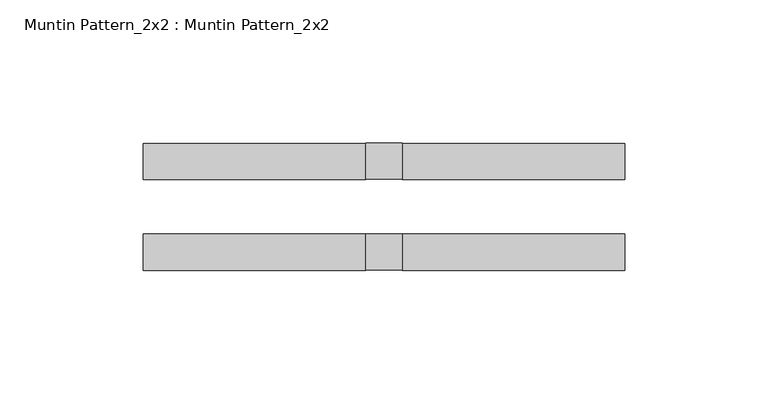
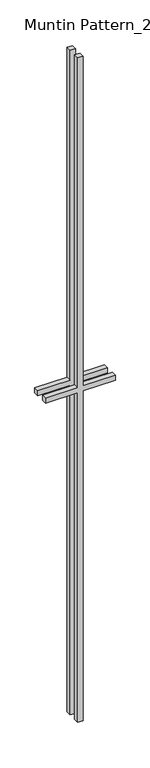
"""IFC4 building model written with IfcOpenShell, lengths in millimetres: proxy geometry, Muntin Pattern_2x2 : Muntin Pattern_2x2."""

from ifc_helpers import new_model, si_unit, frame, origin, place, context, project, spatial, polyline, outline, extrude, source, transform, mapped, element, save


def muntin_pattern_2x2_muntin_pattern_2x2_cdee2e69(model_context):
    return source(origin(), model_context, "Body", "SweptSolid", [
        extrude(outline(polyline([(850.9, -6.35), (850.9, -84.1375), (838.2, -84.1375), (838.2, -6.35), (0.0, -6.35), (0.0, 6.35), (838.2, 6.35), (838.2, 84.1375), (850.9, 84.1375), (850.9, 6.35), (1689.1, 6.35), (1689.1, -6.35), (850.9, -6.35)])), frame((0.0, 9.525, 0.0), z_axis=(0.0, 1.0, 0.0), x_axis=(0.0, 0.0, 1.0)), (0.0, 0.0, 1.0), 12.7),
        extrude(outline(polyline([(850.9, -6.35), (850.9, -84.1375), (838.2, -84.1375), (838.2, -6.35), (0.0, -6.35), (0.0, 6.35), (838.2, 6.35), (838.2, 84.1375), (850.9, 84.1375), (850.9, 6.35), (1689.1, 6.35), (1689.1, -6.35), (850.9, -6.35)])), frame((0.0, -22.225, 0.0), z_axis=(0.0, 1.0, 0.0), x_axis=(0.0, 0.0, 1.0)), (0.0, 0.0, 1.0), 12.7),
    ])


if __name__ == "__main__":
    model = new_model("IFC4")
    model_context = context("Model", 3, world=origin())
    ifc_project = project(units=[si_unit("LENGTHUNIT", "METRE", prefix="MILLI")], contexts=[model_context])
    site = spatial("IfcSite", under=ifc_project)
    building = spatial("IfcBuilding", under=site)
    placement = place(None, origin())
    muntin_pattern_2x2_muntin_pattern_2x2_shape = muntin_pattern_2x2_muntin_pattern_2x2_cdee2e69(model_context)
    element("IfcBuildingElementProxy", 1, Name="Muntin Pattern_2x2 : Muntin Pattern_2x2", ObjectType="Muntin Pattern_2x2 : Muntin Pattern_2x2", at=placement, inside=building, context=model_context, shape_type="MappedRepresentation", body=[
        mapped(muntin_pattern_2x2_muntin_pattern_2x2_shape, transform((0.0, 0.0, 0.0), x_axis=(1.0, 0.0, 0.0), y_axis=(0.0, 1.0, 0.0), z_axis=(0.0, 0.0, 1.0))),
    ])
    save(model, "model.ifc")

# Revit data of these elements
# Type "Muntin Pattern_2x2 : Muntin Pattern_2x2"
#   Width [instance default] = 4' - 0"
#   Thickness = 0' - 0 1/2"
#   Height [instance default] = 4' - 0"
#   Distance = 0' - 0 3/4"
#   Interior Material [instance default] = none
#   Exterior Material [instance default] = none
#   Default Elevation = 0
# Element 1 (IfcBuildingElementProxy, "Muntin Pattern_2x2 : Muntin Pattern_2x2")
#   Width = 0' - 6 5/8"
#   Height = 5' - 6 1/2"
#   Interior Material = Wood - Stained
#   Exterior Material = Clad - White
#   Materials on its faces: "Clad - White", "Wood - Stained"
# Materials
#   "Clad - White": class "Wood", colour RGB 242 242 238, transparency 0, Cost = 0
#   "Wood - Stained": class "Wood", colour RGB 224 178 126, transparency 0, Cost = 0
